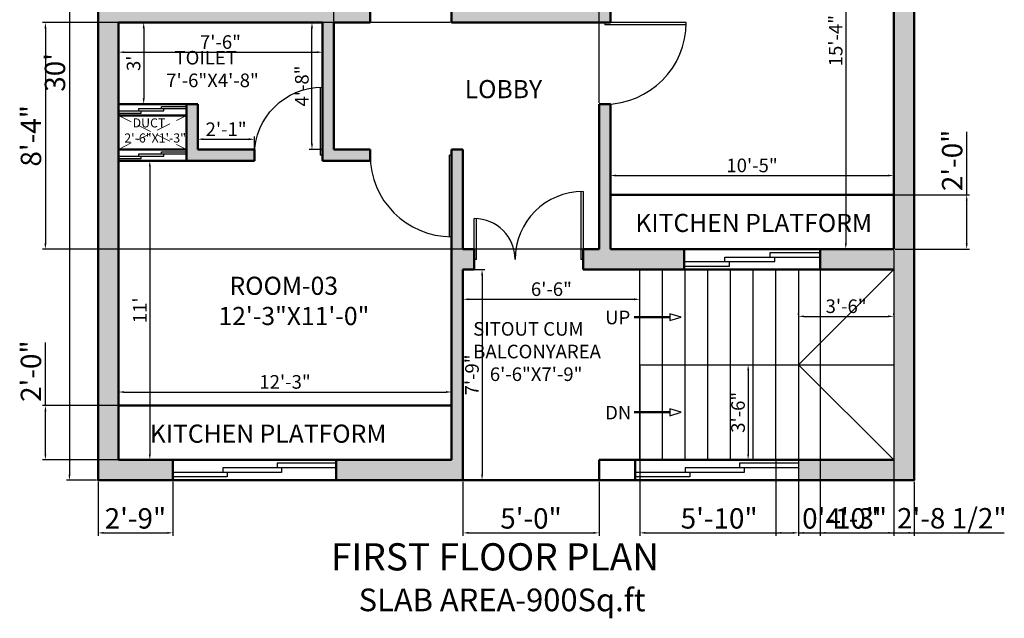
# Model space of a CAD drawing. Units: inches. Extents: x 3274 to 5176, y 1085 to 2172.
# Tile 3 of 16: x 3763 to 4197, y 1118 to 1383. Entities that reach past the tile are written whole.
import ezdxf

# ---------------------------------------------------------------- set-up
doc = ezdxf.new("R2010")
doc.units = ezdxf.units.IN
doc.linetypes.add('DASHED', pattern=[19.05, 12.7, -6.35])
for name, color, linetype, lineweight in [('A-ANNO-DIMS', 2, 'Continuous', 18), ('A-ANNO-TEXT', 7, 'Continuous', 25), ('A-AREA-IDEN', 3, 'Continuous', 25), ('A-DOOR', 4, 'Continuous', 25), ('A-FLOR-OPEN', 7, 'DASHED', 18), ('A-FLOR-STRS', 7, 'Continuous', 25), ('A-GLAZ', 5, 'Continuous', 25), ('A-WALL', 7, 'Continuous', 50), ('A-WALL-PATT', 8, 'Continuous', 13)]:
    doc.layers.add(name, color=color, linetype=linetype, lineweight=lineweight)
doc.styles.get("Standard").update_dxf_attribs({"font": 'arial.ttf'})
doc.dimstyles.new('ISO-25', dxfattribs={"dimtxt": 9, "dimasz": 2.5, "dimexe": 1.25, "dimexo": 0.625, "dimtad": 1, "dimdec": 1, "dimlunit": 3, "dimtxsty": 'Standard', "dimcen": 2.5, "dimclrd": 4, "dimclre": 4, "dimclrt": 1, "dimadec": 0, "dimazin": 0, "dimtfac": 1, "dimtdec": 1, "dimtmove": 0, "dimatfit": 3, "dimfxl": 1, "dimarcsym": 0})

# ---------------------------------------------------------------- blocks, each defined once
blk = doc.blocks.new('*D9')
at = {"layer": 'A-ANNO-DIMS', "color": 0, "lineweight": -2, "transparency": 16777216}
for p, q in [((3797.07, 1539.28), (3783.84, 1539.28)), ((3785.09, 1536.78), (3785.09, 1181.78)), ((3797.07, 1179.28), (3783.84, 1179.28))]:
    blk.add_line(p, q, dxfattribs=at)
at = {"layer": 'A-ANNO-DIMS', "color": 0, "transparency": 16777216}
for points in [[(3784.67, 1536.78), (3785.51, 1536.78), (3785.09, 1539.28)], [(3784.67, 1181.78), (3785.51, 1181.78), (3785.09, 1179.28)]]:
    blk.add_solid(points, dxfattribs=at)
at = {"layer": 'Defpoints', "color": 0, "transparency": 16777216}
for p in [(3797.7, 1539.28), (3785.09, 1179.28), (3797.7, 1179.28)]:
    blk.add_point(p, dxfattribs=at)
at = {"layer": 'A-ANNO-DIMS', "color": 0, "transparency": 16777216, "insert": (3779.87, 1359.28), "char_height": 9, "attachment_point": 5, "rotation": 90}
blk.add_mtext("30'", dxfattribs=at)
blk = doc.blocks.new('3')
for p, q in [((47, 30), (47, 0)), ((48, 30), (48, 0)), ((0, 0), (0, 18)), ((1, 0), (1, 18)), ((1, 0), (0, 0)), ((48, 0), (47, 0))]:
    blk.add_line(p, q)
for centre, radius, start, end in [((48, 0), 30, 90, 180), ((0, 0), 18, 0, 90)]:
    blk.add_arc(centre, radius, start, end)
blk = doc.blocks.new('1')
for p, q in [((0, 36), (0, 0)), ((1, 36), (1, 0)), ((0, 0), (1, 0))]:
    blk.add_line(p, q)
blk.add_arc((0, 0), 36, 0, 90)
blk = doc.blocks.new('2')
for p, q in [((0, 30), (0, 0)), ((1, 30), (1, 0)), ((0, 0), (1, 0))]:
    blk.add_line(p, q)
blk.add_arc((0, 0), 30, 0, 90)
blk = doc.blocks.new('*D36')
at = {"layer": 'A-ANNO-DIMS', "color": 0, "lineweight": -2, "transparency": 16777216}
for p, q in [((3807.32, 1381.28), (3819.09, 1381.28)), ((3817.84, 1378.78), (3817.84, 1347.78)), ((3807.32, 1345.28), (3819.09, 1345.28))]:
    blk.add_line(p, q, dxfattribs=at)
at = {"layer": 'A-ANNO-DIMS', "color": 0, "transparency": 16777216}
for points in [[(3817.42, 1378.78), (3818.26, 1378.78), (3817.84, 1381.28)], [(3817.42, 1347.78), (3818.26, 1347.78), (3817.84, 1345.28)]]:
    blk.add_solid(points, dxfattribs=at)
at = {"layer": 'Defpoints', "color": 0, "transparency": 16777216}
for p in [(3806.7, 1381.28), (3806.7, 1345.28), (3817.84, 1345.28)]:
    blk.add_point(p, dxfattribs=at)
at = {"layer": 'A-ANNO-DIMS', "color": 0, "transparency": 16777216, "insert": (3814.15, 1363.28), "char_height": 6, "attachment_point": 5, "rotation": 90}
blk.add_mtext("3'", dxfattribs=at)
blk = doc.blocks.new('*D37')
at = {"layer": 'A-ANNO-DIMS', "color": 0, "lineweight": -2, "transparency": 16777216}
for p, q in [((3806.7, 1380.66), (3806.7, 1366.94)), ((3896.7, 1375.66), (3896.7, 1366.94)), ((3809.2, 1368.19), (3894.2, 1368.19))]:
    blk.add_line(p, q, dxfattribs=at)
at = {"layer": 'A-ANNO-DIMS', "color": 0, "transparency": 16777216}
for points in [[(3809.2, 1368.61), (3809.2, 1367.78), (3806.7, 1368.19)], [(3894.2, 1368.61), (3894.2, 1367.78), (3896.7, 1368.19)]]:
    blk.add_solid(points, dxfattribs=at)
at = {"layer": 'Defpoints', "color": 0, "transparency": 16777216}
for p in [(3806.7, 1381.28), (3896.7, 1376.28), (3896.7, 1368.19)]:
    blk.add_point(p, dxfattribs=at)
at = {"layer": 'A-ANNO-DIMS', "color": 0, "transparency": 16777216, "insert": (3851.7, 1371.88), "char_height": 6, "attachment_point": 5}
blk.add_mtext('7\'-6"', dxfattribs=at)
blk = doc.blocks.new('*D38')
at = {"layer": 'A-ANNO-DIMS', "color": 0, "lineweight": -2, "transparency": 16777216}
for p, q in [((3841.7, 1325.91), (3841.7, 1331.03)), ((3844.2, 1329.78), (3864.2, 1329.78)), ((3866.7, 1325.91), (3866.7, 1331.03))]:
    blk.add_line(p, q, dxfattribs=at)
at = {"layer": 'A-ANNO-DIMS', "color": 0, "transparency": 16777216}
for points in [[(3844.2, 1330.2), (3844.2, 1329.36), (3841.7, 1329.78)], [(3864.2, 1330.2), (3864.2, 1329.36), (3866.7, 1329.78)]]:
    blk.add_solid(points, dxfattribs=at)
at = {"layer": 'Defpoints', "color": 0, "transparency": 16777216}
for p in [(3866.7, 1329.78), (3841.7, 1325.28), (3866.7, 1325.28)]:
    blk.add_point(p, dxfattribs=at)
at = {"layer": 'A-ANNO-DIMS', "color": 0, "transparency": 16777216, "insert": (3854.2, 1333.42), "char_height": 6, "attachment_point": 5}
blk.add_mtext('2\'-1"', dxfattribs=at)
blk = doc.blocks.new('*D39')
at = {"layer": 'A-ANNO-DIMS', "color": 0, "lineweight": -2, "transparency": 16777216}
for p, q in [((3901.07, 1381.28), (3890.83, 1381.28)), ((3892.08, 1327.78), (3892.08, 1378.78)), ((3896.07, 1325.28), (3890.83, 1325.28))]:
    blk.add_line(p, q, dxfattribs=at)
at = {"layer": 'A-ANNO-DIMS', "color": 0, "transparency": 16777216}
for points in [[(3891.66, 1378.78), (3892.49, 1378.78), (3892.08, 1381.28)], [(3891.66, 1327.78), (3892.49, 1327.78), (3892.08, 1325.28)]]:
    blk.add_solid(points, dxfattribs=at)
at = {"layer": 'Defpoints', "color": 0, "transparency": 16777216}
for p in [(3892.08, 1381.28), (3901.7, 1381.28), (3896.7, 1325.28)]:
    blk.add_point(p, dxfattribs=at)
at = {"layer": 'A-ANNO-DIMS', "color": 0, "transparency": 16777216, "insert": (3888.39, 1353.28), "char_height": 6, "attachment_point": 5, "rotation": 90}
blk.add_mtext('4\'-8"', dxfattribs=at)
blk = doc.blocks.new('*D40')
at = {"layer": 'A-ANNO-DIMS', "color": 0, "lineweight": -2, "transparency": 16777216}
for p, q in [((3807.32, 1320.28), (3821.79, 1320.28)), ((3820.54, 1317.78), (3820.54, 1190.78)), ((3807.32, 1188.28), (3821.79, 1188.28))]:
    blk.add_line(p, q, dxfattribs=at)
at = {"layer": 'A-ANNO-DIMS', "color": 0, "transparency": 16777216}
for points in [[(3820.13, 1317.78), (3820.96, 1317.78), (3820.54, 1320.28)], [(3820.13, 1190.78), (3820.96, 1190.78), (3820.54, 1188.28)]]:
    blk.add_solid(points, dxfattribs=at)
at = {"layer": 'Defpoints', "color": 0, "transparency": 16777216}
for p in [(3806.7, 1320.28), (3806.7, 1188.28), (3820.54, 1188.28)]:
    blk.add_point(p, dxfattribs=at)
at = {"layer": 'A-ANNO-DIMS', "color": 0, "transparency": 16777216, "insert": (3816.91, 1254.28), "char_height": 6, "attachment_point": 5, "rotation": 90}
blk.add_mtext("11'", dxfattribs=at)
blk = doc.blocks.new('*D41')
at = {"layer": 'A-ANNO-DIMS', "color": 0, "lineweight": -2, "transparency": 16777216}
for p, q in [((3806.7, 1212.91), (3806.7, 1219.48)), ((3809.2, 1218.23), (3951.2, 1218.23)), ((3953.7, 1212.91), (3953.7, 1219.48))]:
    blk.add_line(p, q, dxfattribs=at)
at = {"layer": 'A-ANNO-DIMS', "color": 0, "transparency": 16777216}
for points in [[(3809.2, 1218.65), (3809.2, 1217.82), (3806.7, 1218.23)], [(3951.2, 1218.65), (3951.2, 1217.82), (3953.7, 1218.23)]]:
    blk.add_solid(points, dxfattribs=at)
at = {"layer": 'Defpoints', "color": 0, "transparency": 16777216}
for p in [(3953.7, 1218.23), (3806.7, 1212.28), (3953.7, 1212.28)]:
    blk.add_point(p, dxfattribs=at)
at = {"layer": 'A-ANNO-DIMS', "color": 0, "transparency": 16777216, "insert": (3880.2, 1221.92), "char_height": 6, "attachment_point": 5}
blk.add_mtext('12\'-3"', dxfattribs=at)
blk = doc.blocks.new('*D42')
at = {"layer": 'A-ANNO-DIMS', "color": 0, "lineweight": -2, "transparency": 16777216}
for p, q in [((3959.32, 1272.28), (3968.37, 1272.28)), ((3967.12, 1269.78), (3967.12, 1181.78)), ((3959.32, 1179.28), (3968.37, 1179.28))]:
    blk.add_line(p, q, dxfattribs=at)
at = {"layer": 'A-ANNO-DIMS', "color": 0, "transparency": 16777216}
for points in [[(3966.7, 1269.78), (3967.54, 1269.78), (3967.12, 1272.28)], [(3966.7, 1181.78), (3967.54, 1181.78), (3967.12, 1179.28)]]:
    blk.add_solid(points, dxfattribs=at)
at = {"layer": 'Defpoints', "color": 0, "transparency": 16777216}
for p in [(3958.7, 1272.28), (3958.7, 1179.28), (3967.12, 1179.28)]:
    blk.add_point(p, dxfattribs=at)
at = {"layer": 'A-ANNO-DIMS', "color": 0, "transparency": 16777216, "insert": (3963.43, 1225.78), "char_height": 6, "attachment_point": 5, "rotation": 90}
blk.add_mtext('7\'-9"', dxfattribs=at)
blk = doc.blocks.new('*D43')
at = {"layer": 'A-ANNO-DIMS', "color": 0, "lineweight": -2, "transparency": 16777216}
for p, q in [((4036.7, 1259.77), (4036.7, 1260.4)), ((3958.7, 1258.52), (3958.7, 1257.9)), ((3961.2, 1259.15), (4034.2, 1259.15))]:
    blk.add_line(p, q, dxfattribs=at)
at = {"layer": 'A-ANNO-DIMS', "color": 0, "transparency": 16777216}
for points in [[(3961.2, 1259.56), (3961.2, 1258.73), (3958.7, 1259.15)], [(4034.2, 1259.56), (4034.2, 1258.73), (4036.7, 1259.15)]]:
    blk.add_solid(points, dxfattribs=at)
at = {"layer": 'Defpoints', "color": 0, "transparency": 16777216}
for p in [(3958.7, 1259.15), (4036.7, 1259.15), (4036.7, 1259.15)]:
    blk.add_point(p, dxfattribs=at)
at = {"layer": 'A-ANNO-DIMS', "color": 0, "transparency": 16777216, "insert": (3997.7, 1262.84), "char_height": 6, "attachment_point": 5}
blk.add_mtext('6\'-6"', dxfattribs=at)
blk = doc.blocks.new('*D44')
at = {"layer": 'A-ANNO-DIMS', "color": 0, "lineweight": -2, "transparency": 16777216}
for p, q in [((4106.7, 1252.25), (4106.7, 1252.87)), ((4109.2, 1251.62), (4146.2, 1251.62)), ((4148.7, 1252.25), (4148.7, 1252.87))]:
    blk.add_line(p, q, dxfattribs=at)
at = {"layer": 'A-ANNO-DIMS', "color": 0, "transparency": 16777216}
for points in [[(4109.2, 1252.04), (4109.2, 1251.2), (4106.7, 1251.62)], [(4146.2, 1252.04), (4146.2, 1251.2), (4148.7, 1251.62)]]:
    blk.add_solid(points, dxfattribs=at)
at = {"layer": 'Defpoints', "color": 0, "transparency": 16777216}
for p in [(4106.7, 1251.62), (4148.7, 1251.62), (4148.7, 1251.62)]:
    blk.add_point(p, dxfattribs=at)
at = {"layer": 'A-ANNO-DIMS', "color": 0, "transparency": 16777216, "insert": (4127.7, 1255.31), "char_height": 6, "attachment_point": 5}
blk.add_mtext('3\'-6"', dxfattribs=at)
blk = doc.blocks.new('*D45')
at = {"layer": 'A-ANNO-DIMS', "color": 0, "lineweight": -2, "transparency": 16777216}
for p, q in [((4081.81, 1230.28), (4085.74, 1230.28)), ((4084.49, 1227.78), (4084.49, 1190.78)), ((4081.81, 1188.28), (4085.74, 1188.28))]:
    blk.add_line(p, q, dxfattribs=at)
at = {"layer": 'A-ANNO-DIMS', "color": 0, "transparency": 16777216}
for points in [[(4084.08, 1227.78), (4084.91, 1227.78), (4084.49, 1230.28)], [(4084.08, 1190.78), (4084.91, 1190.78), (4084.49, 1188.28)]]:
    blk.add_solid(points, dxfattribs=at)
at = {"layer": 'Defpoints', "color": 0, "transparency": 16777216}
for p in [(4081.18, 1230.28), (4081.18, 1188.28), (4084.49, 1188.28)]:
    blk.add_point(p, dxfattribs=at)
at = {"layer": 'A-ANNO-DIMS', "color": 0, "transparency": 16777216, "insert": (4080.8, 1209.28), "char_height": 6, "attachment_point": 5, "rotation": 90}
blk.add_mtext('3\'-6"', dxfattribs=at)
blk = doc.blocks.new('*D46')
at = {"layer": 'A-ANNO-DIMS', "color": 0, "lineweight": -2, "transparency": 16777216}
for p, q in [((4023.7, 1305.91), (4023.7, 1315)), ((4026.2, 1313.75), (4146.2, 1313.75)), ((4148.7, 1305.91), (4148.7, 1315))]:
    blk.add_line(p, q, dxfattribs=at)
at = {"layer": 'A-ANNO-DIMS', "color": 0, "transparency": 16777216}
for points in [[(4026.2, 1314.17), (4026.2, 1313.34), (4023.7, 1313.75)], [(4146.2, 1314.17), (4146.2, 1313.34), (4148.7, 1313.75)]]:
    blk.add_solid(points, dxfattribs=at)
at = {"layer": 'Defpoints', "color": 0, "transparency": 16777216}
for p in [(4148.7, 1313.75), (4023.7, 1305.28), (4148.7, 1305.28)]:
    blk.add_point(p, dxfattribs=at)
at = {"layer": 'A-ANNO-DIMS', "color": 0, "transparency": 16777216, "insert": (4086.2, 1317.44), "char_height": 6, "attachment_point": 5}
blk.add_mtext('10\'-5"', dxfattribs=at)
blk = doc.blocks.new('*D47')
at = {"layer": 'A-ANNO-DIMS', "color": 0, "lineweight": -2, "transparency": 16777216}
for p, q in [((4113.32, 1465.28), (4128.81, 1465.28)), ((4127.56, 1462.78), (4127.56, 1283.78)), ((4116.82, 1281.28), (4128.81, 1281.28))]:
    blk.add_line(p, q, dxfattribs=at)
at = {"layer": 'A-ANNO-DIMS', "color": 0, "transparency": 16777216}
for points in [[(4127.15, 1462.78), (4127.98, 1462.78), (4127.56, 1465.28)], [(4127.15, 1283.78), (4127.98, 1283.78), (4127.56, 1281.28)]]:
    blk.add_solid(points, dxfattribs=at)
at = {"layer": 'Defpoints', "color": 0, "transparency": 16777216}
for p in [(4112.7, 1465.28), (4116.2, 1281.28), (4127.56, 1281.28)]:
    blk.add_point(p, dxfattribs=at)
at = {"layer": 'A-ANNO-DIMS', "color": 0, "transparency": 16777216, "insert": (4123.87, 1373.28), "char_height": 6, "attachment_point": 5, "rotation": 90}
blk.add_mtext('15\'-4"', dxfattribs=at)
blk = doc.blocks.new('WIN-30')
for p, q in [((4366.19, 1316.35), (4386.19, 1316.35)), ((4375.19, 1317.35), (4396.19, 1317.35)), ((4375.19, 1316.35), (4375.19, 1317.35)), ((4376.19, 1315.35), (4376.19, 1316.35)), ((4385.19, 1318.35), (4396.19, 1318.35)), ((4385.19, 1317.35), (4385.19, 1318.35)), ((4386.19, 1316.35), (4386.19, 1317.35)), ((4366.19, 1315.35), (4376.19, 1315.35))]:
    blk.add_line(p, q)
blk = doc.blocks.new('WIN-60')
for p, q in [((4618.19, 1273.85), (4640.19, 1273.85)), ((4618.19, 1271.85), (4618.19, 1273.85)), ((4580.19, 1269.85), (4620.19, 1269.85)), ((4598.19, 1271.85), (4640.19, 1271.85)), ((4598.19, 1269.85), (4598.19, 1271.85)), ((4600.19, 1267.85), (4600.19, 1269.85)), ((4620.19, 1269.85), (4620.19, 1271.85)), ((4580.19, 1267.85), (4600.19, 1267.85))]:
    blk.add_line(p, q)
blk = doc.blocks.new('WIN-72')
for p, q in [((4462.19, 1178.85), (4412.19, 1178.85)), ((4412.19, 1178.85), (4412.19, 1176.85)), ((4462.19, 1180.85), (4436.19, 1180.85)), ((4436.19, 1180.85), (4436.19, 1178.85)), ((4438.19, 1178.85), (4438.19, 1176.85)), ((4438.19, 1176.85), (4390.19, 1176.85)), ((4414.19, 1174.85), (4390.19, 1174.85)), ((4414.19, 1176.85), (4414.19, 1174.85))]:
    blk.add_line(p, q)
blk = doc.blocks.new('*D192')
at = {"layer": 'A-ANNO-DIMS', "color": 4, "lineweight": -2, "transparency": 16777216}
for p, q in [((3797.7, 1178.66), (3797.7, 1154.83)), ((3830.7, 1178.66), (3830.7, 1154.83)), ((3800.2, 1156.08), (3828.2, 1156.08))]:
    blk.add_line(p, q, dxfattribs=at)
at = {"layer": 'A-ANNO-DIMS', "color": 4, "transparency": 16777216}
for points in [[(3800.2, 1156.5), (3800.2, 1155.66), (3797.7, 1156.08)], [(3828.2, 1156.5), (3828.2, 1155.66), (3830.7, 1156.08)]]:
    blk.add_solid(points, dxfattribs=at)
at = {"layer": 'Defpoints', "color": 0, "transparency": 16777216}
for p in [(3797.7, 1179.28), (3830.7, 1179.28), (3830.7, 1156.08)]:
    blk.add_point(p, dxfattribs=at)
at = {"layer": 'A-ANNO-DIMS', "color": 1, "transparency": 16777216, "insert": (3814.2, 1161.3), "char_height": 9, "attachment_point": 5}
blk.add_mtext('2\'-9"', dxfattribs=at)
blk = doc.blocks.new('*D193')
at = {"layer": 'A-ANNO-DIMS', "color": 4, "lineweight": -2, "transparency": 16777216}
for p, q in [((4106.7, 1178.66), (4106.7, 1154.83)), ((4157.7, 1178.66), (4157.7, 1154.83)), ((4109.2, 1156.08), (4155.2, 1156.08))]:
    blk.add_line(p, q, dxfattribs=at)
at = {"layer": 'A-ANNO-DIMS', "color": 4, "transparency": 16777216}
for points in [[(4109.2, 1156.5), (4109.2, 1155.66), (4106.7, 1156.08)], [(4155.2, 1156.5), (4155.2, 1155.66), (4157.7, 1156.08)]]:
    blk.add_solid(points, dxfattribs=at)
at = {"layer": 'Defpoints', "color": 0, "transparency": 16777216}
for p in [(4106.7, 1179.28), (4157.7, 1179.28), (4157.7, 1156.08)]:
    blk.add_point(p, dxfattribs=at)
at = {"layer": 'A-ANNO-DIMS', "color": 1, "transparency": 16777216, "insert": (4132.2, 1161.3), "char_height": 9, "attachment_point": 5}
blk.add_mtext('4\'-3"', dxfattribs=at)
blk = doc.blocks.new('*D194')
at = {"layer": 'A-ANNO-DIMS', "color": 4, "lineweight": -2, "transparency": 16777216}
for p, q in [((3958.7, 1178.66), (3958.7, 1154.83)), ((4018.7, 1178.66), (4018.7, 1154.83)), ((3961.2, 1156.08), (4016.2, 1156.08))]:
    blk.add_line(p, q, dxfattribs=at)
at = {"layer": 'A-ANNO-DIMS', "color": 4, "transparency": 16777216}
for points in [[(3961.2, 1156.5), (3961.2, 1155.66), (3958.7, 1156.08)], [(4016.2, 1156.5), (4016.2, 1155.66), (4018.7, 1156.08)]]:
    blk.add_solid(points, dxfattribs=at)
at = {"layer": 'Defpoints', "color": 0, "transparency": 16777216}
for p in [(3958.7, 1179.28), (4018.7, 1179.28), (4018.7, 1156.08)]:
    blk.add_point(p, dxfattribs=at)
at = {"layer": 'A-ANNO-DIMS', "color": 1, "transparency": 16777216, "insert": (3988.7, 1161.3), "char_height": 9, "attachment_point": 5}
blk.add_mtext('5\'-0"', dxfattribs=at)
blk = doc.blocks.new('*D195')
at = {"layer": 'A-ANNO-DIMS', "color": 4, "lineweight": -2, "transparency": 16777216}
for p, q in [((3774.5, 1212.28), (3774.5, 1240.11)), ((3953.07, 1212.28), (3773.25, 1212.28)), ((3774.5, 1190.78), (3774.5, 1209.78)), ((3953.07, 1188.28), (3773.25, 1188.28))]:
    blk.add_line(p, q, dxfattribs=at)
at = {"layer": 'A-ANNO-DIMS', "color": 4, "transparency": 16777216}
for points in [[(3774.08, 1209.78), (3774.91, 1209.78), (3774.5, 1212.28)], [(3774.08, 1190.78), (3774.91, 1190.78), (3774.5, 1188.28)]]:
    blk.add_solid(points, dxfattribs=at)
at = {"layer": 'Defpoints', "color": 0, "transparency": 16777216}
for p in [(3774.5, 1212.28), (3953.7, 1212.28), (3953.7, 1188.28)]:
    blk.add_point(p, dxfattribs=at)
at = {"layer": 'A-ANNO-DIMS', "color": 1, "transparency": 16777216, "insert": (3769.27, 1227.45), "char_height": 9, "attachment_point": 5, "rotation": 90}
blk.add_mtext('2\'-0"', dxfattribs=at)
blk = doc.blocks.new('*D197')
at = {"layer": 'A-ANNO-DIMS', "color": 4, "lineweight": -2, "transparency": 16777216}
for p, q in [((4180.9, 1305.28), (4180.9, 1333.11)), ((4149.32, 1305.28), (4182.15, 1305.28)), ((4180.9, 1283.78), (4180.9, 1302.78)), ((4149.32, 1281.28), (4182.15, 1281.28))]:
    blk.add_line(p, q, dxfattribs=at)
at = {"layer": 'A-ANNO-DIMS', "color": 4, "transparency": 16777216}
for points in [[(4180.48, 1302.78), (4181.31, 1302.78), (4180.9, 1305.28)], [(4180.48, 1283.78), (4181.31, 1283.78), (4180.9, 1281.28)]]:
    blk.add_solid(points, dxfattribs=at)
at = {"layer": 'Defpoints', "color": 0, "transparency": 16777216}
for p in [(4148.7, 1305.28), (4180.9, 1305.28), (4148.7, 1281.28)]:
    blk.add_point(p, dxfattribs=at)
at = {"layer": 'A-ANNO-DIMS', "color": 1, "transparency": 16777216, "insert": (4175.67, 1320.45), "char_height": 9, "attachment_point": 5, "rotation": 90}
blk.add_mtext('2\'-0"', dxfattribs=at)
blk = doc.blocks.new('*D198')
at = {"layer": 'A-ANNO-DIMS', "color": 4, "lineweight": -2, "transparency": 16777216}
for p, q in [((4036.7, 1229.66), (4036.7, 1154.83)), ((4106.7, 1229.66), (4106.7, 1154.83)), ((4039.2, 1156.08), (4104.2, 1156.08))]:
    blk.add_line(p, q, dxfattribs=at)
at = {"layer": 'A-ANNO-DIMS', "color": 4, "transparency": 16777216}
for points in [[(4039.2, 1156.5), (4039.2, 1155.66), (4036.7, 1156.08)], [(4104.2, 1156.5), (4104.2, 1155.66), (4106.7, 1156.08)]]:
    blk.add_solid(points, dxfattribs=at)
at = {"layer": 'Defpoints', "color": 0, "transparency": 16777216}
for p in [(4036.7, 1230.28), (4106.7, 1230.28), (4106.7, 1156.08)]:
    blk.add_point(p, dxfattribs=at)
at = {"layer": 'A-ANNO-DIMS', "color": 1, "transparency": 16777216, "insert": (4071.7, 1161.3), "char_height": 9, "attachment_point": 5}
blk.add_mtext('5\'-10"', dxfattribs=at)
blk = doc.blocks.new('*D199')
at = {"layer": 'A-ANNO-DIMS', "color": 4, "lineweight": -2, "transparency": 16777216}
for p, q in [((4096.7, 1187.66), (4096.7, 1154.83)), ((4106.7, 1187.66), (4106.7, 1154.83)), ((4099.2, 1156.08), (4104.2, 1156.08)), ((4106.7, 1156.08), (4141.36, 1156.08))]:
    blk.add_line(p, q, dxfattribs=at)
at = {"layer": 'A-ANNO-DIMS', "color": 4, "transparency": 16777216}
for points in [[(4099.2, 1156.5), (4099.2, 1155.66), (4096.7, 1156.08)], [(4104.2, 1156.5), (4104.2, 1155.66), (4106.7, 1156.08)]]:
    blk.add_solid(points, dxfattribs=at)
at = {"layer": 'Defpoints', "color": 0, "transparency": 16777216}
for p in [(4096.7, 1188.28), (4106.7, 1188.28), (4106.7, 1156.08)]:
    blk.add_point(p, dxfattribs=at)
at = {"layer": 'A-ANNO-DIMS', "color": 1, "transparency": 16777216, "insert": (4125.28, 1161.3), "char_height": 9, "attachment_point": 5}
blk.add_mtext('0\'-10"', dxfattribs=at)
blk = doc.blocks.new('*D200')
at = {"layer": 'A-ANNO-DIMS', "color": 4, "lineweight": -2, "transparency": 16777216}
for p, q in [((3901.7, 1381.91), (3901.7, 1563.73)), ((4018.7, 1345.91), (4018.7, 1563.73)), ((3904.2, 1562.48), (4016.2, 1562.48))]:
    blk.add_line(p, q, dxfattribs=at)
at = {"layer": 'A-ANNO-DIMS', "color": 4, "transparency": 16777216}
for points in [[(3904.2, 1562.9), (3904.2, 1562.06), (3901.7, 1562.48)], [(4016.2, 1562.9), (4016.2, 1562.06), (4018.7, 1562.48)]]:
    blk.add_solid(points, dxfattribs=at)
at = {"layer": 'Defpoints', "color": 0, "transparency": 16777216}
for p in [(4018.7, 1562.48), (3901.7, 1381.28), (4018.7, 1345.28)]:
    blk.add_point(p, dxfattribs=at)
at = {"layer": 'A-ANNO-DIMS', "color": 1, "transparency": 16777216, "insert": (3960.2, 1567.7), "char_height": 9, "attachment_point": 5}
blk.add_mtext('9\'-9"', dxfattribs=at)
blk = doc.blocks.new('*D201')
at = {"layer": 'A-ANNO-DIMS', "color": 4, "lineweight": -2, "transparency": 16777216}
for p, q in [((3953.07, 1381.28), (3773.25, 1381.28)), ((3774.5, 1378.78), (3774.5, 1283.78)), ((4018.07, 1281.28), (3773.25, 1281.28))]:
    blk.add_line(p, q, dxfattribs=at)
at = {"layer": 'A-ANNO-DIMS', "color": 4, "transparency": 16777216}
for points in [[(3774.08, 1378.78), (3774.91, 1378.78), (3774.5, 1381.28)], [(3774.08, 1283.78), (3774.91, 1283.78), (3774.5, 1281.28)]]:
    blk.add_solid(points, dxfattribs=at)
at = {"layer": 'Defpoints', "color": 0, "transparency": 16777216}
for p in [(3953.7, 1381.28), (3774.5, 1281.28), (4018.7, 1281.28)]:
    blk.add_point(p, dxfattribs=at)
at = {"layer": 'A-ANNO-DIMS', "color": 1, "transparency": 16777216, "insert": (3769.27, 1331.28), "char_height": 9, "attachment_point": 5, "rotation": 90}
blk.add_mtext('8\'-4"', dxfattribs=at)
blk = doc.blocks.new('*D202')
at = {"layer": 'A-ANNO-DIMS', "color": 4, "lineweight": -2, "transparency": 16777216}
for p, q in [((4116.2, 1280.66), (4116.2, 1154.83)), ((4148.7, 1280.66), (4148.7, 1154.83)), ((4118.7, 1156.08), (4146.2, 1156.08)), ((4148.7, 1156.08), (4197.49, 1156.08))]:
    blk.add_line(p, q, dxfattribs=at)
at = {"layer": 'A-ANNO-DIMS', "color": 4, "transparency": 16777216}
for points in [[(4118.7, 1156.5), (4118.7, 1155.66), (4116.2, 1156.08)], [(4146.2, 1156.5), (4146.2, 1155.66), (4148.7, 1156.08)]]:
    blk.add_solid(points, dxfattribs=at)
at = {"layer": 'Defpoints', "color": 0, "transparency": 16777216}
for p in [(4116.2, 1281.28), (4148.7, 1281.28), (4148.7, 1156.08)]:
    blk.add_point(p, dxfattribs=at)
at = {"layer": 'A-ANNO-DIMS', "color": 1, "transparency": 16777216, "insert": (4174.34, 1161.36), "char_height": 9, "attachment_point": 5}
blk.add_mtext('2\'-8 1/2"', dxfattribs=at)

msp = doc.modelspace()

# ---------------------------------------------------------------- hatches: boundary and pattern name
at = {"layer": 'A-WALL-PATT'}
h = msp.add_hatch(color=256, dxfattribs=at)
h.dxf.hatch_style = 1
h.paths.add_polyline_path([(3958.7, 1489.28), (3976.7, 1489.28), (3976.7, 1494.28), (3953.7, 1494.28), (3953.7, 1454.28), (3958.7, 1454.28)], flags=17)
h.paths.add_polyline_path([(4023.7, 1494.28), (4000.7, 1494.28), (4000.7, 1489.28), (4018.7, 1489.28), (4018.7, 1386.28), (3958.7, 1386.28), (3958.7, 1424.28), (3956.2, 1424.28), (3953.7, 1424.28), (3953.7, 1381.28), (4023.7, 1381.28), (4023.7, 1465.28), (4112.7, 1465.28), (4112.7, 1470.28), (4023.7, 1470.28)], flags=17)
h.paths.add_polyline_path([(4056.2, 1281.28), (4023.7, 1281.28), (4023.7, 1345.28), (4018.7, 1345.28), (4018.7, 1281.28), (4011.7, 1281.28), (4011.7, 1276.78), (4011.7, 1272.28), (4056.2, 1272.28)], flags=17)
h.paths.add_polyline_path([(3963.7, 1281.28), (3958.7, 1281.28), (3958.7, 1325.28), (3953.7, 1325.28), (3953.7, 1188.28), (3902.7, 1188.28), (3902.7, 1179.28), (3958.7, 1179.28), (3958.7, 1272.28), (3963.7, 1272.28)], flags=17)
h.paths.add_polyline_path([(3806.7, 1530.28), (4107.7, 1530.28), (4107.7, 1500.28), (4112.7, 1500.28), (4112.7, 1530.28), (4148.7, 1530.28), (4148.7, 1281.28), (4116.2, 1281.28), (4116.2, 1272.28), (4148.7, 1272.28), (4148.7, 1188.28), (4106.7, 1188.28), (4106.7, 1179.28), (4157.7, 1179.28), (4157.7, 1539.28), (3797.7, 1539.28), (3797.7, 1179.28), (3830.7, 1179.28), (3830.7, 1188.28), (3806.7, 1188.28), (3806.7, 1381.28), (3896.7, 1381.28), (3896.7, 1320.28), (3917.7, 1320.28), (3917.7, 1325.28), (3901.7, 1325.28), (3901.7, 1381.28), (3917.7, 1381.28), (3917.7, 1386.28), (3806.7, 1386.28)])
h.paths.add_polyline_path([(3866.7, 1325.28), (3841.7, 1325.28), (3841.7, 1345.28), (3836.7, 1345.28), (3836.7, 1320.28), (3866.7, 1320.28)], flags=17)
h.paths.add_polyline_path([(4115.78, 1513.99), (4148.63, 1513.99), (4148.63, 1528.42), (4115.78, 1528.42)], flags=25)
h.paths.add_polyline_path([(3961.09, 1219.59), (4026.99, 1219.59), (4026.99, 1252.09), (3961.09, 1252.09)], flags=25)
h.paths.add_polyline_path([(3956.63, 1343.39), (3997.9, 1343.39), (3997.9, 1359.88), (3956.63, 1359.88)], flags=25)
h.paths.add_polyline_path([(3817.73, 1191.34), (3934.74, 1191.34), (3934.74, 1207.83), (3817.73, 1207.83)], flags=25)
h.paths.add_polyline_path([(3817.73, 1509.34), (3934.74, 1509.34), (3934.74, 1525.83), (3817.73, 1525.83)], flags=25)
h.paths.add_polyline_path([(4061.81, 1383.87), (4130.2, 1383.87), (4130.2, 1413.72), (4061.81, 1413.72)], flags=25)
h.paths.add_polyline_path([(3847.58, 1243.23), (3915.98, 1243.23), (3915.98, 1273.08), (3847.58, 1273.08)], flags=25)
h.paths.add_polyline_path([(4044.62, 1493.29), (4086.59, 1493.29), (4086.59, 1515.68), (4044.62, 1515.68)], flags=25)
h.paths.add_polyline_path([(3968.18, 1502.97), (4010.15, 1502.97), (4010.15, 1525.36), (3968.18, 1525.36)], flags=25)
h.paths.add_polyline_path([(3969.86, 1456.15), (4011.83, 1456.15), (4011.83, 1478.54), (3969.86, 1478.54)], flags=24)
h.paths.add_polyline_path([(3847.58, 1449.68), (3915.98, 1449.68), (3915.98, 1479.54), (3847.58, 1479.54)], flags=25)
h.paths.add_polyline_path([(4019.88, 1246.5), (4034.58, 1246.5), (4034.58, 1255.65), (4019.88, 1255.65)], flags=25)
h.paths.add_polyline_path([(4019.91, 1204.63), (4035.01, 1204.63), (4035.01, 1213.63), (4019.91, 1213.63)], flags=25)
h.paths.add_polyline_path([(3825.87, 1349.35), (3867.84, 1349.35), (3867.84, 1371.74), (3825.87, 1371.74)], flags=25)

# ---------------------------------------------------------------- linework, layer by layer
at = {"layer": 'A-FLOR-OPEN', "ltscale": 0.5}
for p, q in [((3806.7, 1340.28), (3836.7, 1325.28)), ((3806.7, 1325.28), (3836.7, 1340.28))]:
    msp.add_line(p, q, dxfattribs=at)
at = {"layer": 'A-FLOR-STRS'}
for p, q in [((4036.7, 1230.28), (4036.7, 1272.28)), ((4046.7, 1230.28), (4046.7, 1272.28)), ((4056.7, 1230.28), (4056.7, 1272.28)), ((4066.7, 1230.28), (4066.7, 1272.28)), ((4076.7, 1230.28), (4076.7, 1272.28)), ((4086.7, 1230.28), (4086.7, 1272.28)), ((4096.7, 1230.28), (4096.7, 1272.28)), ((4106.7, 1272.28), (4106.7, 1188.28)), ((4106.7, 1230.28), (4148.7, 1272.28)), ((4148.7, 1272.28), (4148.7, 1188.28)), ((4036.7, 1230.28), (4148.7, 1230.28)), ((4036.7, 1188.28), (4036.7, 1230.28)), ((4046.7, 1188.28), (4046.7, 1230.28)), ((4056.7, 1188.28), (4056.7, 1230.28)), ((4066.7, 1188.28), (4066.7, 1230.28)), ((4076.7, 1188.28), (4076.7, 1230.28)), ((4086.7, 1188.28), (4086.7, 1230.28)), ((4096.7, 1188.28), (4096.7, 1230.28)), ((4106.7, 1230.28), (4148.7, 1188.28)), ((4106.7, 1188.28), (4106.7, 1179.28))]:
    msp.add_line(p, q, dxfattribs=at)
for points in [[(4054.9, 1251.28), (4050.01, 1252.78), (4050.01, 1249.78)], [(4054.9, 1209.28), (4050.01, 1210.78), (4050.01, 1207.78)]]:
    msp.add_lwpolyline(points, close=True, dxfattribs=at)
at = {"layer": 'A-WALL'}
for p, q in [((4148.7, 1530.28), (4148.7, 1281.28)), ((4023.7, 1465.28), (4023.7, 1381.28)), ((3953.7, 1381.28), (3953.7, 1424.28)), ((3917.7, 1381.28), (3917.7, 1386.28)), ((3806.7, 1381.28), (3896.7, 1381.28)), ((3806.7, 1188.28), (3806.7, 1381.28)), ((3896.7, 1320.28), (3896.7, 1381.28)), ((3901.7, 1325.28), (3901.7, 1381.28)), ((3901.7, 1381.28), (3917.7, 1381.28)), ((3953.7, 1381.28), (4023.7, 1381.28)), ((3806.7, 1345.28), (3841.7, 1345.28)), ((3836.7, 1320.28), (3836.7, 1345.28)), ((3841.7, 1325.28), (3841.7, 1345.28)), ((4018.7, 1345.28), (4023.7, 1345.28)), ((4018.7, 1345.28), (4018.7, 1281.28)), ((4023.7, 1345.28), (4023.7, 1281.28)), ((3806.7, 1340.28), (3836.7, 1340.28)), ((3806.7, 1325.28), (3836.7, 1325.28)), ((3841.7, 1325.28), (3866.7, 1325.28)), ((3866.7, 1320.28), (3866.7, 1325.28)), ((3901.7, 1325.28), (3917.7, 1325.28)), ((3917.7, 1320.28), (3917.7, 1325.28)), ((3953.7, 1325.28), (3958.7, 1325.28)), ((3953.7, 1188.28), (3953.7, 1325.28)), ((3958.7, 1281.28), (3958.7, 1325.28)), ((3806.7, 1320.28), (3866.7, 1320.28)), ((3896.7, 1320.28), (3917.7, 1320.28)), ((4023.7, 1305.28), (4148.7, 1305.28)), ((3958.7, 1281.28), (3963.7, 1281.28)), ((3963.7, 1272.28), (3963.7, 1281.28)), ((4011.7, 1281.28), (4018.7, 1281.28)), ((4011.7, 1272.28), (4011.7, 1281.28)), ((4023.7, 1281.28), (4148.7, 1281.28)), ((4056.2, 1272.28), (4056.2, 1281.28)), ((4116.2, 1272.28), (4116.2, 1281.28)), ((3958.7, 1272.28), (3963.7, 1272.28)), ((3958.7, 1179.28), (3958.7, 1272.28)), ((4011.7, 1272.28), (4148.7, 1272.28)), ((4034.25, 1251.28), (4050.01, 1251.28)), ((3953.7, 1212.28), (3806.7, 1212.28)), ((4034.25, 1209.28), (4050.01, 1209.28)), ((3953.7, 1188.28), (3806.7, 1188.28)), ((3830.7, 1188.28), (3830.7, 1179.28)), ((3902.7, 1188.28), (3902.7, 1179.28)), ((4148.7, 1188.28), (4018.7, 1188.28)), ((4018.7, 1179.28), (4018.7, 1188.28)), ((4034.7, 1188.28), (4034.7, 1179.28))]:
    msp.add_line(p, q, dxfattribs=at)
msp.add_lwpolyline([(3958.7, 1179.28), (3797.7, 1179.28), (3797.7, 1539.28), (4157.7, 1539.28), (4157.7, 1179.28), (3958.7, 1179.28)], dxfattribs=at)

# ---------------------------------------------------------------- block references
at = {"layer": 'A-DOOR'}
for p, rotation in [((4021.2, 1381.28), 270), ((3953.7, 1322.78), 180)]:
    msp.add_blockref('1', p, dxfattribs=dict(at, rotation=rotation))
at = {"layer": 'A-DOOR', "xscale": -1}
msp.add_blockref('2', (3896.7, 1322.78), dxfattribs=at)
at = {"layer": 'A-DOOR'}
msp.add_blockref('3', (3963.7, 1276.78), dxfattribs=at)
at = {"layer": 'A-GLAZ'}
for name, p in [('WIN-30', (-559.49, 25.93)), ('WIN-30', (-559.49, 5.93)), ('WIN-60', (-523.99, 5.93)), ('WIN-72', (-559.49, 5.93)), ('WIN-72', (-355.49, 5.93))]:
    msp.add_blockref(name, p, dxfattribs=at)

# ---------------------------------------------------------------- texts
at = {"layer": 'A-ANNO-TEXT'}
for s, p in [('UP', (4021.41, 1248.13)), ('DN', (4021.41, 1206.13))]:
    msp.add_text(s, height=6, dxfattribs=at).set_placement(p)
at = {"layer": 'A-ANNO-TEXT', "insert": (3900.43, 1151.5), "char_height": 12, "attachment_point": 1}
msp.add_mtext_dynamic_manual_height_columns('FIRST FLOOR PLAN\\P{\\H0.83333x;    SLAB AREA-900Sq.ft}', width=202.3193, gutter_width=30, heights=[0], dxfattribs=at)
at = {"layer": 'A-AREA-IDEN', "attachment_point": 1}
for s, width, heights, insert, char_height in [('  TOILET\\P7\'-6"X4\'-8"', 58.0121, [16.24], (3827.77, 1368.76), 6), ('LOBBY', 58.0121, [16.24], (3959.44, 1355.9), 8), ('   DUCT\\P2\'-6"X1\'-3"', 58.0121, [16.24], (3809.29, 1338.99), 4), ('KITCHEN PLATFORM', 147.1149, [0], (4034.75, 1296.85), 8), ('  ROOM-03\\P12\'-3"X11\'-0"', 58.0121, [0], (3850.8, 1269.11), 8), ('SITOUT CUM BALCONYAREA \\P    6\'-6"X7\'-9"', 58.0121, [0], (3963.2, 1249.1), 6), ('KITCHEN PLATFORM', 147.1149, [0], (3820.54, 1203.85), 8)]:
    msp.add_mtext_dynamic_manual_height_columns(s, width=width, gutter_width=30, heights=heights, dxfattribs=dict(at, insert=insert, char_height=char_height))

# ---------------------------------------------------------------- dimensions: what is measured, and where the dimension line sits
at = {"layer": 'A-ANNO-DIMS'}
for base, p1, p2, override, picture, middle in [((4018.7, 1562.48), (3901.7, 1381.28), (4018.7, 1345.28), {"dimdec": 1, "dimlfac": 1, "dimrnd": 0, "dimzin": 1, "dimdsep": 46, "dimlunit": 4, "dimfrac": 2}, '*D200', (3960.2, 1567.7)), ((3896.7, 1368.19), (3806.7, 1381.28), (3896.7, 1376.28), {"dimtxt": 6, "dimclrd": 0, "dimclre": 0, "dimclrt": 0}, '*D37', (3851.7, 1371.88)), ((3866.7, 1329.78), (3841.7, 1325.28), (3866.7, 1325.28), {"dimtxt": 6, "dimclrd": 0, "dimclre": 0, "dimclrt": 0}, '*D38', (3854.2, 1333.42)), ((4148.7, 1313.75), (4023.7, 1305.28), (4148.7, 1305.28), {"dimtxt": 6, "dimclrd": 0, "dimclre": 0, "dimclrt": 0}, '*D46', (4086.2, 1317.44)), ((4148.7, 1156.08), (4116.2, 1281.28), (4148.7, 1281.28), {"dimdec": 1, "dimlfac": 1, "dimrnd": 0, "dimzin": 1, "dimdsep": 46, "dimlunit": 4, "dimfrac": 2}, '*D202', (4174.34, 1161.36)), ((4036.7, 1259.15), (3958.7, 1259.15), (4036.7, 1259.15), {"dimtxt": 6, "dimclrd": 0, "dimclre": 0, "dimclrt": 0}, '*D43', (3997.7, 1262.84)), ((4148.7, 1251.62), (4106.7, 1251.62), (4148.7, 1251.62), {"dimtxt": 6, "dimclrd": 0, "dimclre": 0, "dimclrt": 0}, '*D44', (4127.7, 1255.31)), ((4106.7, 1156.08), (4036.7, 1230.28), (4106.7, 1230.28), {"dimdec": 1, "dimlfac": 1, "dimrnd": 0, "dimzin": 1, "dimdsep": 46, "dimlunit": 4, "dimfrac": 2}, '*D198', (4071.7, 1161.3)), ((3953.7, 1218.23), (3806.7, 1212.28), (3953.7, 1212.28), {"dimtxt": 6, "dimclrd": 0, "dimclre": 0, "dimclrt": 0}, '*D41', (3880.2, 1221.92)), ((4106.7, 1156.08), (4096.7, 1188.28), (4106.7, 1188.28), {"dimdec": 1, "dimlfac": 1, "dimrnd": 0, "dimzin": 1, "dimdsep": 46, "dimlunit": 4, "dimfrac": 2}, '*D199', (4125.28, 1161.3)), ((3830.7, 1156.08), (3797.7, 1179.28), (3830.7, 1179.28), {"dimdec": 1, "dimlfac": 1, "dimrnd": 0, "dimzin": 1, "dimdsep": 46, "dimlunit": 4, "dimfrac": 2}, '*D192', (3814.2, 1161.3)), ((4018.7, 1156.08), (3958.7, 1179.28), (4018.7, 1179.28), {"dimdec": 1, "dimlfac": 1, "dimrnd": 0, "dimzin": 1, "dimdsep": 46, "dimlunit": 4, "dimfrac": 2}, '*D194', (3988.7, 1161.3)), ((4157.7, 1156.08), (4106.7, 1179.28), (4157.7, 1179.28), {"dimdec": 1, "dimlfac": 1, "dimrnd": 0, "dimzin": 1, "dimdsep": 46, "dimlunit": 4, "dimfrac": 2}, '*D193', (4132.2, 1161.3))]:
    dim = msp.add_linear_dim(base=base, p1=p1, p2=p2, dimstyle='ISO-25', override=override, dxfattribs=at)
    dim.commit()
    dim.dimension.update_dxf_attribs({"geometry": picture, "text_midpoint": middle})
for base, p1, p2, override, picture, middle in [((3785.09, 1179.28), (3797.7, 1539.28), (3797.7, 1179.28), {"dimclrd": 0, "dimclre": 0, "dimclrt": 0}, '*D9', (3779.87, 1359.28)), ((4127.56, 1281.28), (4112.7, 1465.28), (4116.2, 1281.28), {"dimtxt": 6, "dimclrd": 0, "dimclre": 0, "dimclrt": 0}, '*D47', (4123.87, 1373.28)), ((3774.5, 1281.28), (3953.7, 1381.28), (4018.7, 1281.28), {"dimdec": 1, "dimlfac": 1, "dimrnd": 0, "dimzin": 1, "dimdsep": 46, "dimlunit": 4, "dimfrac": 2}, '*D201', (3769.27, 1331.28)), ((3817.84, 1345.28), (3806.7, 1381.28), (3806.7, 1345.28), {"dimtxt": 6, "dimclrd": 0, "dimclre": 0, "dimclrt": 0}, '*D36', (3814.15, 1363.28)), ((3892.08, 1381.28), (3896.7, 1325.28), (3901.7, 1381.28), {"dimtxt": 6, "dimclrd": 0, "dimclre": 0, "dimclrt": 0}, '*D39', (3888.39, 1353.28)), ((4180.9, 1305.28), (4148.7, 1281.28), (4148.7, 1305.28), {"dimdec": 1, "dimlfac": 1, "dimrnd": 0, "dimzin": 1, "dimdsep": 46, "dimlunit": 4, "dimfrac": 2}, '*D197', (4175.67, 1320.45)), ((3820.54, 1188.28), (3806.7, 1320.28), (3806.7, 1188.28), {"dimtxt": 6, "dimclrd": 0, "dimclre": 0, "dimclrt": 0}, '*D40', (3816.91, 1254.28)), ((3967.12, 1179.28), (3958.7, 1272.28), (3958.7, 1179.28), {"dimtxt": 6, "dimclrd": 0, "dimclre": 0, "dimclrt": 0}, '*D42', (3963.43, 1225.78)), ((3774.5, 1212.28), (3953.7, 1188.28), (3953.7, 1212.28), {"dimdec": 1, "dimlfac": 1, "dimrnd": 0, "dimzin": 1, "dimdsep": 46, "dimlunit": 4, "dimfrac": 2}, '*D195', (3769.27, 1227.45)), ((4084.49, 1188.28), (4081.18, 1230.28), (4081.18, 1188.28), {"dimtxt": 6, "dimclrd": 0, "dimclre": 0, "dimclrt": 0}, '*D45', (4080.8, 1209.28))]:
    dim = msp.add_linear_dim(base=base, p1=p1, p2=p2, angle=90, dimstyle='ISO-25', override=override, dxfattribs=at)
    dim.commit()
    dim.dimension.update_dxf_attribs({"geometry": picture, "text_midpoint": middle})

doc.saveas('drawing.dxf')
